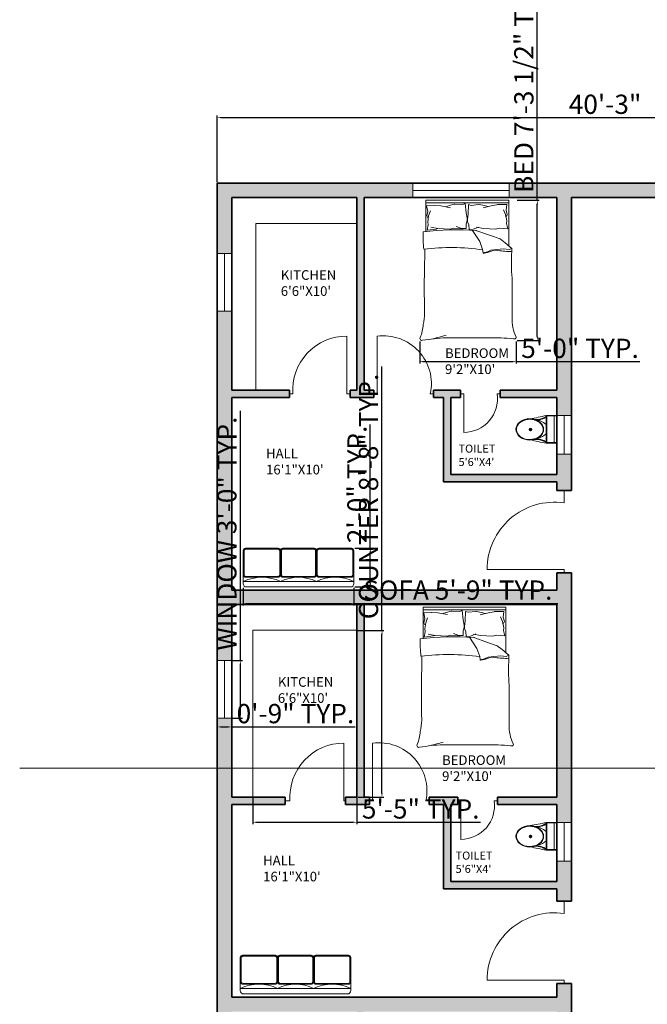
# Model space of a CAD drawing. Units: inches. Extents: x 1266 to 2869, y -408 to 3241.
# Tile 8 of 11: x 2029 to 2420, y 1767 to 2380. Entities that reach past the tile are written whole.
import ezdxf

# ---------------------------------------------------------------- set-up
doc = ezdxf.new("R2010")
doc.units = ezdxf.units.IN
for name, color, linetype, lineweight in [('A-ANNO-DIMS', 2, 'Continuous', 18), ('A-ANNO-SYMB', 7, 'Continuous', 18), ('A-AREA-IDEN', 7, 'Continuous', 18), ('A-DOOR', 4, 'Continuous', 18), ('A-FLOR-CASE', 9, 'Continuous', 18), ('A-FLOR-FIXT', 9, 'Continuous', 18), ('A-FURN', 8, 'Continuous', 18), ('A-GLAZ', 4, 'Continuous', 18), ('A-WALL', 7, 'Continuous', 35), ('A-WALL-PATT', 251, 'Continuous', 13)]:
    doc.layers.add(name, color=color, linetype=linetype, lineweight=lineweight)
doc.styles.get("Standard").update_dxf_attribs({"font": 'arial.ttf'})
doc.dimstyles.new('ISO-25', dxfattribs={"dimtxt": 12, "dimasz": 2.5, "dimexe": 1.25, "dimexo": 0.625, "dimtad": 1, "dimdec": 0, "dimlunit": 3, "dimtxsty": 'Standard', "dimcen": 2.5, "dimadec": 0, "dimazin": 0, "dimtfac": 1, "dimtdec": 0, "dimtmove": 0, "dimatfit": 3, "dimfxl": 1, "dimarcsym": 0})

# ---------------------------------------------------------------- blocks, each defined once
blk = doc.blocks.new('A$C31115884')
for p, q in [((283, 498), (223, 498)), ((258, 466), (258, 523)), ((0, 200), (0, 0)), ((520, 200), (0, 200)), ((10, 190), (10, 10)), ((510, 190), (10, 190)), ((510, 10), (510, 190)), ((520, 0), (520, 200)), ((510, 54), (0, 54)), ((10, 10), (510, 10)), ((0, 0), (520, 0))]:
    blk.add_line(p, q)
blk.add_circle((256, 496), 23.6)
for centre, radius, start, end in [((2778, -205), 2807, 165.4549, 171.7133), ((-295, 403), 365, 324.2091, 9.3499), ((-295, 403), 375, 324.2091, 9.3499), ((139, 406), 293, 315.8436, 2.6563), ((806, 403), 375, 179.2036, 215.7909), ((806, 403), 365, 170.6501, 215.7909), ((3237, 905), 2807, 188.2867, 194.5451), ((384, 406), 293, 190.2774, 224.1564)]:
    blk.add_arc(centre, radius, start, end)
blk.add_ellipse((256, 510), major_axis=(0, -261), ratio=0.772727)
blk.add_open_spline([(256, 259), (263, 259), (270, 260), (288, 262), (299, 265), (320, 273), (330, 278), (350, 291), (360, 299), (378, 316), (386, 326), (402, 347), (409, 358), (421, 383), (427, 395), (436, 422), (440, 436), (445, 465), (447, 480), (448, 509), (448, 524), (445, 553), (443, 568), (436, 596), (432, 610), (422, 636), (416, 649), (402, 672), (395, 683), (379, 703), (370, 712), (351, 728), (341, 735), (321, 746), (310, 751), (289, 757), (278, 759), (256, 761), (245, 761), (223, 757), (212, 754), (191, 746), (181, 741), (161, 728), (151, 720), (133, 703), (125, 693), (110, 672), (103, 660), (90, 636), (85, 623), (76, 596), (72, 582), (67, 553), (66, 538), (64, 509), (65, 494), (68, 465), (70, 450), (77, 422), (81, 408), (91, 382), (97, 370), (111, 346), (118, 335), (135, 316), (144, 307), (162, 291), (172, 284), (193, 273), (203, 269), (225, 262), (236, 260), (250, 259), (253, 259), (256, 259)], degree=3, knots=[0, 0, 0, 0, 0.110105, 0.110105, 0.285049, 0.285049, 0.459994, 0.459994, 0.634938, 0.634938, 0.809882, 0.809882, 0.984827, 0.984827, 1.159771, 1.159771, 1.334715, 1.334715, 1.50966, 1.50966, 1.684604, 1.684604, 1.859549, 1.859549, 2.034493, 2.034493, 2.209437, 2.209437, 2.384382, 2.384382, 2.559326, 2.559326, 2.73427, 2.73427, 2.909215, 2.909215, 3.084159, 3.084159, 3.259103, 3.259103, 3.434048, 3.434048, 3.608992, 3.608992, 3.783936, 3.783936, 3.958881, 3.958881, 4.133825, 4.133825, 4.30877, 4.30877, 4.483714, 4.483714, 4.658658, 4.658658, 4.833603, 4.833603, 5.008547, 5.008547, 5.183491, 5.183491, 5.358436, 5.358436, 5.53338, 5.53338, 5.708324, 5.708324, 5.883269, 5.883269, 6.058213, 6.058213, 6.233158, 6.233158, 6.283185, 6.283185, 6.283185, 6.283185])
blk = doc.blocks.new('*D4')
at = {"layer": 'A-ANNO-DIMS', "color": 0, "lineweight": -2, "transparency": 16777216}
for p, q in [((2152.45, 2278.97), (2152.45, 2320.42)), ((2154.95, 2319.17), (2632.95, 2319.17)), ((2635.45, 2278.97), (2635.45, 2320.42))]:
    blk.add_line(p, q, dxfattribs=at)
at = {"layer": 'A-ANNO-DIMS', "color": 0, "transparency": 16777216}
for points in [[(2154.95, 2319.59), (2154.95, 2318.76), (2152.45, 2319.17)], [(2632.95, 2319.59), (2632.95, 2318.76), (2635.45, 2319.17)]]:
    blk.add_solid(points, dxfattribs=at)
at = {"layer": 'Defpoints', "color": 0, "transparency": 16777216}
for p in [(2635.45, 2319.17), (2152.45, 2278.35), (2635.45, 2278.35)]:
    blk.add_point(p, dxfattribs=at)
at = {"layer": 'A-ANNO-DIMS', "color": 0, "transparency": 16777216, "insert": (2393.95, 2325.93), "char_height": 12, "attachment_point": 5}
blk.add_mtext('40\'-3"', dxfattribs=at)
blk = doc.blocks.new('BED-DOUBLE')
for p, q in [((3.76, 67.77), (3.76, 87.35)), ((3.76, 87.35), (55.42, 87.35)), ((55.42, 87.35), (55.42, 58.59)), ((3.76, 85.69), (55.42, 85.69)), ((4.21, 83.74), (8.84, 84.1)), ((4.21, 83.77), (4.84, 80.33)), ((4.84, 80.33), (4.37, 77.51)), ((5.46, 77.67), (6.55, 80.64)), ((8.84, 84.1), (8.96, 84.08)), ((8.96, 84.08), (13.09, 83.77)), ((13.09, 83.77), (19.03, 82.67)), ((16.06, 83.3), (18.25, 84.08)), ((18.25, 84.08), (21.37, 84.86)), ((21.37, 84.86), (21.72, 84.86)), ((21.72, 84.86), (26.53, 84.7)), ((26.53, 84.7), (28.09, 85.33)), ((28.09, 85.33), (28.71, 79.55)), ((30.24, 84.66), (29.98, 78.85)), ((31.84, 84.13), (30.24, 84.66)), ((36.63, 84.59), (31.84, 84.13)), ((36.98, 84.61), (36.63, 84.59)), ((40.14, 84.02), (36.98, 84.61)), ((45.31, 84.03), (39.45, 82.57)), ((42.38, 83.38), (40.14, 84.02)), ((49.42, 84.6), (45.31, 84.03)), ((54.17, 84.59), (48.33, 84.69)), ((48.33, 84.69), (49.42, 84.6)), ((53.3, 78.43), (52.03, 81.32)), ((54.17, 84.59), (53.76, 81.12)), ((53.76, 81.12), (54.41, 78.34)), ((4.37, 77.51), (4.99, 76.42)), ((4.84, 73.76), (5.46, 77.67)), ((5.15, 72.04), (4.84, 73.76)), ((28.71, 79.55), (29.34, 76.11)), ((29.34, 74.7), (28.71, 72.67)), ((29.34, 76.11), (29.34, 74.7)), ((29.98, 78.85), (29.57, 75.38)), ((29.57, 75.38), (29.66, 73.97)), ((29.66, 73.97), (30.41, 71.98)), ((54.17, 74.56), (53.3, 78.43)), ((54.41, 78.34), (53.85, 77.21)), ((53.97, 72.83), (54.17, 74.56)), ((4.52, 68.61), (5.15, 72.04)), ((10.03, 69.39), (4.52, 68.61)), ((6.9, 70.46), (11.26, 69.74)), ((11.26, 69.74), (10.03, 69.39)), ((11.26, 69.74), (18.84, 69.27)), ((18.84, 69.27), (20.95, 69.87)), ((20.95, 69.87), (26.5, 69.44)), ((26.06, 69.77), (22.66, 70.95)), ((28.71, 69.77), (26.06, 69.77)), ((28.71, 72.67), (28.71, 69.77)), ((30.41, 71.98), (30.59, 69.09)), ((30.59, 69.09), (33.24, 69.26)), ((32.71, 68.56), (37.24, 61.54)), ((33.24, 69.26), (36.56, 70.64)), ((43.94, 65.39), (34.92, 68.56)), ((35.2, 70.46), (39.56, 69.74)), ((39.56, 69.74), (47.14, 69.27)), ((47.14, 69.27), (49.26, 69.87)), ((49.26, 69.87), (54.81, 69.44)), ((54.81, 69.44), (53.97, 72.83)), ((37.24, 61.54), (39.08, 56.69)), ((49.96, 63.21), (43.94, 65.39)), ((53.15, 60.87), (49.96, 63.21)), ((39.08, 56.69), (39.42, 54.51)), ((42.1, 55.18), (44.27, 56.19)), ((44.27, 56.19), (47.96, 56.69)), ((47.96, 56.69), (52.14, 57.02)), ((52.14, 57.02), (55.49, 56.69)), ((57.15, 57.36), (53.15, 60.87)), ((55.49, 56.69), (57.15, 57.36)), ((57.24, 55.47), (57.15, 57.36, 4.18)), ((39.42, 54.51), (42.1, 55.18)), ((16.28, 1.69), (42.89, 1.69))]:
    blk.add_line(p, q)
for centre, radius, start, end in [((92.06, 65.63), 90.06, 178.72178, 185.60397), ((23.09, -109.45), 178.34, 86.08655, 96.78213), ((19.19, -81.63), 139.47, 81.78449, 96.90062), ((-180.86, 53.65), 183.89, 358.4762, 1.00819), ((33.68, 85.75), 32.06, 280.66171, 289.88058), ((47.29, 49.44), 6.73, 78.6608, 113.73842), ((55.49, 94.55), 39.11, 259.87628, 272.56571), ((197.03, 48.09), 139.99, 176.97912, 183.83645), ((39.6, 54.45), 0.199, 160.24637, 271.13765), ((524.11, 32.64), 521.39, 178.22771, 181.71854), ((-4874.07, 14.03), 4931.49, 0.00217, 0.28689), ((-29.08, 17.61), 32.04, 346.06484, 358.91125), ((82.33, 13.12), 24.93, 177.47136, 206.46809), ((-23.41, 11.38), 25.47, 337.97508, 356.652), ((1.18, 1.17), 1.18, 146.17358, 293.47814), ((23.16, -129.76), 131.62, 92.99578, 99.40907), ((-18.62, 112.98), 115.08, 283.38322, 287.70533), ((44.49, -142.13), 143.82, 84.4998, 90.63509), ((58.82, 2.09), 1.19, 242.65876, 356.02002)]:
    blk.add_arc(centre, radius, start, end)
blk = doc.blocks.new('SOFA-3-SEAT-2')
for points in [[(0, 22.36), (0, 7.74, 0.414214), (1.72, 6.02), (21.5, 6.02, 0.414214), (23.22, 7.74), (23.22, 22.36, 0.414214), (21.5, 24.08), (1.72, 24.08, 0.414214)], [(0.52, 22.36), (0.52, 7.74, 0.414214), (1.72, 6.53), (21.5, 6.53, 0.414214), (22.7, 7.74), (22.7, 22.36, 0.414214), (21.5, 23.56), (1.72, 23.56, 0.414214)], [(45.57, 22.36), (45.57, 7.74, -0.414214), (43.85, 6.02), (24.94, 6.02, -0.414214), (23.22, 7.74), (23.22, 22.36, -0.414214), (24.94, 24.08), (43.85, 24.08, -0.414214)], [(45.06, 22.36), (45.06, 7.74, -0.414214), (43.85, 6.53), (24.94, 6.53, -0.414214), (23.73, 7.74), (23.73, 22.36, -0.414214), (24.94, 23.56), (43.85, 23.56, -0.414214)], [(45.57, 22.36), (45.57, 7.74, 0.414214), (47.29, 6.02), (67.07, 6.02, 0.414214), (68.79, 7.74), (68.79, 22.36, 0.414214), (67.07, 24.08), (47.29, 24.08, 0.414214)], [(46.09, 22.36), (46.09, 7.74, 0.414214), (47.29, 6.53), (67.07, 6.53, 0.414214), (68.27, 7.74), (68.27, 22.36, 0.414214), (67.07, 23.56), (47.29, 23.56, 0.414214)]]:
    blk.add_lwpolyline(points, format="xyb", close=True)
at = {"ltscale": 0.03}
blk.add_lwpolyline([(21.82, 24.08), (1.38, 24.08, 0.414214), (0, 22.7), (0, 2.06, 0.414214), (2.06, 0), (66.73, 0, 0.414214), (68.79, 2.06), (68.79, 22.7, 0.414214), (67.41, 24.08), (46.97, 24.08, 0.414214), (45.59, 22.7, -1), (45.56, 22.7, 0.414214), (44.18, 24.08), (24.61, 24.08, 0.414214), (23.23, 22.7, -1), (23.2, 22.7, 0.414214)], format="xyb", close=True, dxfattribs=at)
blk.add_lwpolyline([(0, 3.44), (68.79, 3.44)])
for centre, radius, start, end in [((11.61, -21.35), 27.38, 64.91063, 115.08937), ((34.4, -19.35), 25.38, 63.869, 116.131), ((57.18, -21.07), 27.12, 64.65382, 115.34618)]:
    blk.add_arc(centre, radius, start, end)
blk = doc.blocks.new('DOOR-KITCHEN-L')
for p, q in [((35.61, 0), (35.61, 36)), ((0, 0), (2, 0)), ((37.61, 0), (35.61, 0))]:
    blk.add_line(p, q)
blk.add_arc((35.61, 2.31), 33.69, 90, 183.92625)
blk = doc.blocks.new('DOOR-BEDROOM-L')
for p, q in [((2, 0), (2, 36)), ((0, 0), (2, 0)), ((37.12, 0.11), (35.12, 0.11))]:
    blk.add_line(p, q)
blk.add_arc((5.98, 6.45), 29.82, 347.72217, 97.67592)
blk = doc.blocks.new('DOOR-BATH-L')
for p, q in [((0, 24), (2, 24)), ((2, 24), (2, 0)), ((24.7, 24), (22.7, 24))]:
    blk.add_line(p, q)
blk.add_arc((2, 20.92), 20.92, 270, 8.45113)
blk = doc.blocks.new('DOOR-ENTRY-L')
for p, q in [((48, 51.27), (48, 45.59)), ((48, 45.59), (48, 43.59)), ((12, 2), (0, 2)), ((48, 2), (12, 2)), ((48, 0), (48, 2))]:
    blk.add_line(p, q)
blk.add_arc((42.02, 2), 42.02, 81.81164, 180)
blk = doc.blocks.new('WIN-PLAN-60')
for p, q in [((0, 9), (0, 0)), ((60, 4.5), (60, 9)), ((60, 9), (60, 0)), ((0, 4.5), (60, 4.5)), ((0, 0), (0, 4.5))]:
    blk.add_line(p, q)
blk = doc.blocks.new('WIN-PLAN-36')
for p, q in [((0, 36), (9, 36)), ((4.5, 36), (4.5, 0)), ((9, 36), (4.5, 36)), ((4.5, 0), (0, 0)), ((0, 0), (9, 0))]:
    blk.add_line(p, q)
blk = doc.blocks.new('WIN-PLAN-36-2')
for p, q in [((0, 36), (9, 36)), ((4.5, 36), (4.5, 0)), ((9, 36), (4.5, 36)), ((2.69, 0), (0, 0)), ((0, 0), (9, 0))]:
    blk.add_line(p, q)
blk = doc.blocks.new('WIN-PLAN-24-2')
for p, q in [((0, 24), (9, 24)), ((4.5, 24), (4.5, 0)), ((9, 24), (4.5, 24)), ((4.5, 0), (0, 0)), ((0, 0), (9, 0))]:
    blk.add_line(p, q)
blk = doc.blocks.new('WIN-PLAN-24-3')
for p, q in [((0, 24), (9, 24)), ((4.5, 24), (4.5, 0)), ((9, 24), (4.5, 24)), ((2.69, 0), (0, 0)), ((0, 0), (9, 0))]:
    blk.add_line(p, q)
blk = doc.blocks.new('COUNTER-KITCHEN-2')
for p, q in [((0, 0), (0, 103.95)), ((0, 103.95), (63, 103.95))]:
    blk.add_line(p, q)
blk = doc.blocks.new('COUNTER-KITCHEN-3')
for p, q in [((0, 0), (0, 103.95)), ((0, 103.95), (64.81, 103.95))]:
    blk.add_line(p, q)
blk = doc.blocks.new('*D39')
at = {"layer": 'A-ANNO-DIMS', "color": 0, "lineweight": -2, "transparency": 16777216}
for p, q in [((2351.77, 2267.74), (2351.77, 2411.2)), ((2339.28, 2267.74), (2353.02, 2267.74)), ((2351.77, 2182.78), (2351.77, 2265.24)), ((2339.28, 2180.28), (2353.02, 2180.28))]:
    blk.add_line(p, q, dxfattribs=at)
at = {"layer": 'A-ANNO-DIMS', "color": 0, "transparency": 16777216}
for points in [[(2351.36, 2265.24), (2352.19, 2265.24), (2351.77, 2267.74)], [(2351.36, 2182.78), (2352.19, 2182.78), (2351.77, 2180.28)]]:
    blk.add_solid(points, dxfattribs=at)
at = {"layer": 'Defpoints', "color": 0, "transparency": 16777216}
for p in [(2338.65, 2267.74), (2351.77, 2267.74), (2338.65, 2180.28)]:
    blk.add_point(p, dxfattribs=at)
at = {"layer": 'A-ANNO-DIMS', "color": 0, "transparency": 16777216, "insert": (2344.94, 2340.72), "char_height": 12, "attachment_point": 5, "rotation": 90}
blk.add_mtext('BED 7\'-3 1/2" TYP.', dxfattribs=at)
blk = doc.blocks.new('*D40')
at = {"layer": 'A-ANNO-DIMS', "color": 0, "lineweight": -2, "transparency": 16777216}
for p, q in [((2278.55, 2179.65), (2278.55, 2165.91)), ((2338.65, 2179.65), (2338.65, 2165.91)), ((2281.05, 2167.16), (2336.15, 2167.16)), ((2338.65, 2167.16), (2415.55, 2167.16))]:
    blk.add_line(p, q, dxfattribs=at)
at = {"layer": 'A-ANNO-DIMS', "color": 0, "transparency": 16777216}
for points in [[(2281.05, 2167.58), (2281.05, 2166.74), (2278.55, 2167.16)], [(2336.15, 2167.58), (2336.15, 2166.74), (2338.65, 2167.16)]]:
    blk.add_solid(points, dxfattribs=at)
at = {"layer": 'Defpoints', "color": 0, "transparency": 16777216}
for p in [(2278.55, 2180.28), (2338.65, 2180.28), (2338.65, 2167.16)]:
    blk.add_point(p, dxfattribs=at)
at = {"layer": 'A-ANNO-DIMS', "color": 0, "transparency": 16777216, "insert": (2378.35, 2173.91), "char_height": 12, "attachment_point": 5}
blk.add_mtext('5\'-0" TYP.', dxfattribs=at)
blk = doc.blocks.new('*D69')
at = {"layer": 'A-ANNO-DIMS', "color": 0, "lineweight": -2, "transparency": 16777216}
for p, q in [((2168.66, 2026.17), (2168.66, 2015.23)), ((2237.45, 2026.17), (2237.45, 2015.23)), ((2171.16, 2016.48), (2234.95, 2016.48)), ((2237.45, 2016.48), (2364.59, 2016.48))]:
    blk.add_line(p, q, dxfattribs=at)
at = {"layer": 'A-ANNO-DIMS', "color": 0, "transparency": 16777216}
for points in [[(2171.16, 2016.9), (2171.16, 2016.06), (2168.66, 2016.48)], [(2234.95, 2016.9), (2234.95, 2016.06), (2237.45, 2016.48)]]:
    blk.add_solid(points, dxfattribs=at)
at = {"layer": 'Defpoints', "color": 0, "transparency": 16777216}
for p in [(2168.66, 2026.8), (2237.45, 2026.8), (2237.45, 2016.48)]:
    blk.add_point(p, dxfattribs=at)
at = {"layer": 'A-ANNO-DIMS', "color": 0, "transparency": 16777216, "insert": (2302.27, 2023.31), "char_height": 12, "attachment_point": 5}
blk.add_mtext('SOFA 5\'-9" TYP.', dxfattribs=at)
blk = doc.blocks.new('*D70')
at = {"layer": 'A-ANNO-DIMS', "color": 0, "lineweight": -2, "transparency": 16777216}
for p, q in [((2247.77, 2050.88), (2247.77, 2127.98)), ((2238.07, 2050.88), (2249.02, 2050.88)), ((2247.77, 2029.3), (2247.77, 2048.38)), ((2238.07, 2026.8), (2249.02, 2026.8))]:
    blk.add_line(p, q, dxfattribs=at)
at = {"layer": 'A-ANNO-DIMS', "color": 0, "transparency": 16777216}
for points in [[(2247.35, 2048.38), (2248.18, 2048.38), (2247.77, 2050.88)], [(2247.35, 2029.3), (2248.18, 2029.3), (2247.77, 2026.8)]]:
    blk.add_solid(points, dxfattribs=at)
at = {"layer": 'Defpoints', "color": 0, "transparency": 16777216}
for p in [(2237.45, 2050.88), (2247.77, 2050.88), (2237.45, 2026.8)]:
    blk.add_point(p, dxfattribs=at)
at = {"layer": 'A-ANNO-DIMS', "color": 0, "transparency": 16777216, "insert": (2241.02, 2090.68), "char_height": 12, "attachment_point": 5, "rotation": 90}
blk.add_mtext('2\'-0" TYP.', dxfattribs=at)
blk = doc.blocks.new('*D75')
at = {"layer": 'A-ANNO-DIMS', "color": 0, "lineweight": -2, "transparency": 16777216}
for p, q in [((2166.85, 1981.02), (2166.85, 2136.62)), ((2162.08, 1981.02), (2168.1, 1981.02)), ((2166.85, 1947.52), (2166.85, 1978.52)), ((2162.08, 1945.02), (2168.1, 1945.02))]:
    blk.add_line(p, q, dxfattribs=at)
at = {"layer": 'A-ANNO-DIMS', "color": 0, "transparency": 16777216}
for points in [[(2166.43, 1978.52), (2167.27, 1978.52), (2166.85, 1981.02)], [(2166.43, 1947.52), (2167.27, 1947.52), (2166.85, 1945.02)]]:
    blk.add_solid(points, dxfattribs=at)
at = {"layer": 'Defpoints', "color": 0, "transparency": 16777216}
for p in [(2161.45, 1981.02), (2166.85, 1981.02), (2161.45, 1945.02)]:
    blk.add_point(p, dxfattribs=at)
at = {"layer": 'A-ANNO-DIMS', "color": 0, "transparency": 16777216, "insert": (2160.01, 2060.07), "char_height": 12, "attachment_point": 5, "rotation": 90}
blk.add_mtext('WINDOW 3\'-0" TYP.', dxfattribs=at)
blk = doc.blocks.new('*D76')
at = {"layer": 'A-ANNO-DIMS', "color": 0, "lineweight": -2, "transparency": 16777216}
for p, q in [((2152.45, 1944.4), (2152.45, 1938.37)), ((2161.45, 1944.4), (2161.45, 1938.37)), ((2154.95, 1939.62), (2158.95, 1939.62)), ((2161.45, 1939.62), (2238.35, 1939.62))]:
    blk.add_line(p, q, dxfattribs=at)
at = {"layer": 'A-ANNO-DIMS', "color": 0, "transparency": 16777216}
for points in [[(2154.95, 1940.04), (2154.95, 1939.21), (2152.45, 1939.62)], [(2158.95, 1940.04), (2158.95, 1939.21), (2161.45, 1939.62)]]:
    blk.add_solid(points, dxfattribs=at)
at = {"layer": 'Defpoints', "color": 0, "transparency": 16777216}
for p in [(2152.45, 1945.02), (2161.45, 1945.02), (2161.45, 1939.62)]:
    blk.add_point(p, dxfattribs=at)
at = {"layer": 'A-ANNO-DIMS', "color": 0, "transparency": 16777216, "insert": (2201.15, 1946.38), "char_height": 12, "attachment_point": 5}
blk.add_mtext('0\'-9" TYP.', dxfattribs=at)
blk = doc.blocks.new('*D79')
at = {"layer": 'A-ANNO-DIMS', "color": 0, "lineweight": -2, "transparency": 16777216}
for p, q in [((2255.04, 1999.79), (2255.04, 2164.1)), ((2240.08, 1999.79), (2256.29, 1999.79)), ((2255.04, 1898.35), (2255.04, 1997.29)), ((2240.08, 1895.85), (2256.29, 1895.85))]:
    blk.add_line(p, q, dxfattribs=at)
at = {"layer": 'A-ANNO-DIMS', "color": 0, "transparency": 16777216}
for points in [[(2254.63, 1997.29), (2255.46, 1997.29), (2255.04, 1999.79)], [(2254.63, 1898.35), (2255.46, 1898.35), (2255.04, 1895.85)]]:
    blk.add_solid(points, dxfattribs=at)
at = {"layer": 'Defpoints', "color": 0, "transparency": 16777216}
for p in [(2239.45, 1999.79), (2255.04, 1999.79), (2239.45, 1895.85)]:
    blk.add_point(p, dxfattribs=at)
at = {"layer": 'A-ANNO-DIMS', "color": 0, "transparency": 16777216, "insert": (2248.21, 2083.2), "char_height": 12, "attachment_point": 5, "rotation": 90}
blk.add_mtext('COUNTER 8\'-8" TYP.', dxfattribs=at)
blk = doc.blocks.new('*D80')
at = {"layer": 'A-ANNO-DIMS', "color": 0, "lineweight": -2, "transparency": 16777216}
for p, q in [((2174.64, 1895.22), (2174.64, 1879)), ((2239.45, 1895.22), (2239.45, 1879)), ((2177.14, 1880.25), (2236.95, 1880.25)), ((2239.45, 1880.25), (2316.35, 1880.25))]:
    blk.add_line(p, q, dxfattribs=at)
at = {"layer": 'A-ANNO-DIMS', "color": 0, "transparency": 16777216}
for points in [[(2177.14, 1880.67), (2177.14, 1879.84), (2174.64, 1880.25)], [(2236.95, 1880.67), (2236.95, 1879.84), (2239.45, 1880.25)]]:
    blk.add_solid(points, dxfattribs=at)
at = {"layer": 'Defpoints', "color": 0, "transparency": 16777216}
for p in [(2174.64, 1895.85), (2239.45, 1895.85), (2239.45, 1880.25)]:
    blk.add_point(p, dxfattribs=at)
at = {"layer": 'A-ANNO-DIMS', "color": 0, "transparency": 16777216, "insert": (2279.15, 1886.98), "char_height": 12, "attachment_point": 5}
blk.add_mtext('5\'-5" TYP.', dxfattribs=at)

msp = doc.modelspace()

# ---------------------------------------------------------------- hatches: boundary and pattern name
at = {"layer": 'A-WALL-PATT'}
h = msp.add_hatch(color=256, dxfattribs=at)
h.dxf.hatch_style = 1
h.paths.add_polyline_path([(2161.45, 2269.35), (2239.45, 2269.35), (2239.45, 2149.35), (2235.18, 2149.35), (2235.18, 2144.85), (2243.95, 2144.85), (2249.99, 2144.85), (2249.99, 2146.74), (2249.99, 2149.35), (2243.95, 2149.35), (2243.95, 2269.35), (2274.21, 2269.35), (2274.21, 2273.85), (2274.21, 2278.35), (2152.45, 2278.35), (2152.45, 2234.52), (2161.45, 2234.52)])
h.paths.add_polyline_path([(2550.01, 2278.35), (2424.95, 2278.35), (2372.95, 2278.35), (2334.21, 2278.35), (2334.21, 2269.35), (2363.95, 2269.35), (2363.95, 2149.35), (2328.7, 2149.35), (2328.7, 2144.85), (2363.95, 2144.85), (2363.95, 2133.61), (2372.95, 2133.61), (2372.95, 2269.35), (2424.95, 2269.35), (2424.95, 2234.52), (2433.95, 2234.52), (2433.95, 2269.35), (2511.95, 2269.35), (2511.95, 2149.35), (2504.09, 2149.35), (2504.09, 2144.85), (2520.49, 2144.85), (2520.49, 2149.35), (2516.45, 2149.35), (2516.45, 2269.35), (2550.01, 2269.35), (2550.01, 2273.85)])
h.paths.add_polyline_path([(2635.45, 2278.35), (2610.01, 2278.35), (2610.01, 2269.35), (2626.45, 2269.35), (2626.45, 2149.35), (2588.98, 2149.35), (2588.98, 2144.85), (2626.45, 2144.85), (2626.45, 2133.61), (2635.45, 2133.61)])
h.paths.add_polyline_path([(2560.45, 2144.85), (2565.84, 2144.85), (2565.84, 2149.35), (2552.33, 2149.35), (2552.33, 2144.85), (2555.95, 2144.85), (2555.95, 2092.35), (2626.45, 2092.35), (2626.45, 2086.89), (2626.45, 2024.85), (2610.01, 2024.85), (2610.01, 2015.85), (2626.45, 2015.85), (2626.45, 1895.85), (2589.21, 1895.85), (2589.21, 1891.35), (2626.45, 1891.35), (2626.45, 1880.11), (2635.45, 1880.11), (2635.45, 2086.89), (2635.45, 2109.61), (2626.45, 2109.61), (2626.45, 2096.85), (2560.45, 2096.85)])
h.paths.add_polyline_path([(2433.95, 2198.52), (2424.95, 2198.52), (2424.95, 2086.89), (2433.95, 2086.89), (2433.95, 2144.85), (2470.3, 2144.85), (2470.3, 2149.35), (2433.95, 2149.35)])
h.paths.add_polyline_path([(2372.95, 2109.61), (2363.95, 2109.61), (2363.95, 2096.85), (2297.95, 2096.85), (2297.95, 2144.85), (2304, 2144.85), (2304, 2149.35), (2293.45, 2149.35), (2287.11, 2149.35), (2287.11, 2144.85), (2293.45, 2144.85), (2293.45, 2092.35), (2363.95, 2092.35), (2363.95, 2086.89), (2372.95, 2086.89)], flags=17)
h.paths.add_polyline_path([(2161.45, 2144.85), (2197.56, 2144.85), (2197.56, 2149.35), (2161.45, 2149.35), (2161.45, 2198.52), (2152.45, 2198.52), (2152.45, 1981.02), (2161.45, 1981.02), (2161.45, 2015.85), (2363.95, 2015.85), (2363.95, 1895.85), (2326.89, 1895.85), (2326.89, 1891.35), (2363.95, 1891.35), (2363.95, 1880.11), (2372.95, 1880.11), (2372.95, 2035.62), (2363.95, 2035.62), (2363.95, 2024.85), (2161.45, 2024.85)])
h.paths.add_polyline_path([(2161.45, 1691.52), (2152.45, 1691.52), (2152.45, 1474.02), (2161.45, 1474.02)])
h.paths.add_polyline_path([(2194.79, 1895.85), (2161.45, 1895.85), (2161.45, 1945.02), (2152.45, 1945.02), (2152.45, 1727.52), (2161.45, 1727.52), (2161.45, 1762.35), (2363.95, 1762.35), (2363.95, 1642.35), (2328.7, 1642.35), (2328.7, 1637.85), (2363.95, 1637.85), (2363.95, 1589.85), (2297.95, 1589.85), (2297.95, 1637.85), (2303.95, 1637.85), (2303.95, 1642.35), (2287.64, 1642.35), (2287.64, 1637.85), (2293.45, 1637.85), (2293.45, 1585.35), (2363.95, 1585.35), (2363.95, 1579.45), (2372.95, 1579.45), (2372.95, 1779.84), (2363.95, 1779.84), (2363.95, 1771.35), (2161.45, 1771.35), (2161.45, 1891.35), (2194.79, 1891.35)])
h.paths.add_polyline_path([(2243.95, 2015.85), (2239.45, 2015.85), (2239.45, 1895.85), (2232.4, 1895.85), (2232.4, 1891.35), (2247.22, 1891.35), (2247.22, 1895.85), (2243.95, 1895.85)], flags=17)
h.paths.add_polyline_path([(2302.19, 1895.85), (2284.34, 1895.85), (2284.34, 1891.35), (2293.45, 1891.35), (2293.45, 1838.85), (2363.95, 1838.85), (2363.95, 1831.11), (2372.95, 1831.11), (2372.95, 1856.11), (2363.95, 1856.11), (2363.95, 1843.35), (2297.95, 1843.35), (2297.95, 1891.35), (2302.19, 1891.35)], flags=17)
h.paths.add_polyline_path([(2243.95, 1762.35), (2239.45, 1762.35), (2239.45, 1642.35), (2235.18, 1642.35), (2235.18, 1637.85), (2249.99, 1637.85), (2249.99, 1642.35), (2243.95, 1642.35)], flags=17)
h.paths.add_polyline_path([(2197.56, 1642.35), (2161.45, 1642.35), (2161.45, 1637.85), (2197.56, 1637.85)], flags=17)
h.paths.add_polyline_path([(2363.95, 1517.85), (2161.45, 1517.85), (2161.45, 1508.85), (2239.45, 1508.85), (2239.45, 1388.85), (2243.95, 1388.85), (2243.95, 1508.85), (2363.95, 1508.85)])
h.paths.add_polyline_path([(2372.95, 1528.18), (2363.95, 1528.18), (2363.95, 1323.21), (2372.95, 1323.21)])
h.paths.add_polyline_path([(2372.95, 1271.94), (2363.95, 1271.94), (2363.95, 1264.35), (2161.45, 1264.35), (2161.45, 1283.77), (2156.95, 1283.77), (2152.45, 1283.77), (2152.45, 1255.35), (2156.95, 1255.35), (2372.95, 1255.35)])
h.paths.add_polyline_path([(2161.45, 1438.02), (2152.45, 1438.02), (2152.45, 1319.77), (2161.45, 1319.77)])
h.paths.add_polyline_path([(2550.01, 1513.35), (2550.01, 1517.85), (2433.95, 1517.85), (2433.95, 1528.62), (2424.95, 1528.62), (2424.95, 1474.02), (2433.95, 1474.02), (2433.95, 1508.85), (2511.95, 1508.85), (2511.95, 1388.85), (2504.09, 1388.85), (2504.09, 1384.35), (2520.49, 1384.35), (2520.49, 1388.85), (2516.45, 1388.85), (2516.45, 1508.85), (2550.01, 1508.85)])
h.paths.add_polyline_path([(2635.45, 1602.61), (2626.45, 1602.61), (2626.45, 1517.85), (2610.01, 1517.85), (2610.01, 1508.85), (2626.45, 1508.85), (2626.45, 1388.85), (2588.98, 1388.85), (2588.98, 1384.35), (2626.45, 1384.35), (2626.45, 1373.11), (2635.45, 1373.11)])
h.paths.add_polyline_path([(2635.45, 1349.11), (2626.45, 1349.11), (2626.45, 1336.35), (2560.45, 1336.35), (2560.45, 1384.35), (2565.84, 1384.35), (2565.84, 1388.85), (2552.33, 1388.85), (2552.33, 1384.35), (2555.95, 1384.35), (2555.95, 1331.85), (2626.45, 1331.85), (2626.45, 1315.59), (2635.45, 1315.59)])
h.paths.add_polyline_path([(2635.45, 1279.59), (2630.95, 1279.59), (2626.45, 1279.59), (2626.45, 1264.35), (2433.95, 1264.35), (2433.95, 1275.12), (2424.95, 1275.12), (2424.95, 1255.35), (2635.45, 1255.35)])
h.paths.add_polyline_path([(2433.95, 1438.02), (2424.95, 1438.02), (2424.95, 1326.39), (2433.95, 1326.39)])
h.paths.add_polyline_path([(2470.3, 1388.85), (2433.95, 1388.85), (2433.95, 1384.35), (2470.3, 1384.35)], flags=0)

# ---------------------------------------------------------------- linework, layer by layer
at = {"layer": 'A-ANNO-SYMB'}
msp.add_line((2029.46, 1914.02), (2745.24, 1914.02), dxfattribs=at)
at = {"layer": 'A-DOOR'}
for p, q in [((2231.36, 1893.6), (2231.36, 1929.6)), ((2194.79, 1893.6), (2196.79, 1893.6)), ((2195.75, 1893.6), (2197.75, 1893.6)), ((2232.4, 1893.6), (2231.36, 1893.6)), ((2232.4, 1893.6), (2231.36, 1893.6))]:
    msp.add_line(p, q, dxfattribs=at)
msp.add_arc((2231.36, 1895.9), 33.69, 90, 183.92625, dxfattribs=at)
at = {"layer": 'A-FURN'}
for points in [[(2166.84, 1795.66), (2166.84, 1781.04, 0.414214), (2168.56, 1779.32), (2188.34, 1779.32, 0.414214), (2190.06, 1781.04), (2190.06, 1795.66, 0.414214), (2188.34, 1797.38), (2168.56, 1797.38, 0.414214)], [(2212.42, 1795.66), (2212.42, 1781.04, -0.414214), (2210.7, 1779.32), (2191.78, 1779.32, -0.414214), (2190.06, 1781.04), (2190.06, 1795.66, -0.414214), (2191.78, 1797.38), (2210.7, 1797.38, -0.414214)], [(2212.42, 1795.66), (2212.42, 1781.04, 0.414214), (2214.14, 1779.32), (2233.92, 1779.32, 0.414214), (2235.63, 1781.04), (2235.63, 1795.66, 0.414214), (2233.92, 1797.38), (2214.14, 1797.38, 0.414214)], [(2167.36, 1795.66), (2167.36, 1781.04, 0.414214), (2168.56, 1779.83), (2188.34, 1779.83, 0.414214), (2189.55, 1781.04), (2189.55, 1795.66, 0.414214), (2188.34, 1796.86), (2168.56, 1796.86, 0.414214)], [(2211.9, 1795.66), (2211.9, 1781.04, -0.414214), (2210.7, 1779.83), (2191.78, 1779.83, -0.414214), (2190.58, 1781.04), (2190.58, 1795.66, -0.414214), (2191.78, 1796.86), (2210.7, 1796.86, -0.414214)], [(2212.93, 1795.66), (2212.93, 1781.04, 0.414214), (2214.14, 1779.83), (2233.92, 1779.83, 0.414214), (2235.12, 1781.04), (2235.12, 1795.66, 0.414214), (2233.92, 1796.86), (2214.14, 1796.86, 0.414214)]]:
    msp.add_lwpolyline(points, format="xyb", close=True, dxfattribs=at)
at = {"layer": 'A-FURN', "ltscale": 0.03}
msp.add_lwpolyline([(2188.67, 1797.38), (2168.22, 1797.38, 0.414214), (2166.84, 1796), (2166.84, 1775.36, 0.414214), (2168.91, 1773.3), (2233.57, 1773.3, 0.414214), (2235.63, 1775.36), (2235.63, 1796, 0.414214), (2234.26, 1797.38), (2213.81, 1797.38, 0.414214), (2212.43, 1796, -1), (2212.4, 1796, 0.414214), (2211.03, 1797.38), (2191.45, 1797.38, 0.414214), (2190.08, 1796, -1), (2190.04, 1796, 0.414214)], format="xyb", close=True, dxfattribs=at)
at = {"layer": 'A-FURN'}
msp.add_lwpolyline([(2166.84, 1776.74), (2235.63, 1776.74)], dxfattribs=at)
for centre, radius, start, end in [((2178.45, 1751.95), 27.38, 64.91063, 115.08937), ((2201.24, 1753.95), 25.38, 63.869, 116.131), ((2224.03, 1752.23), 27.12, 64.65382, 115.34618)]:
    msp.add_arc(centre, radius, start, end, dxfattribs=at)
at = {"layer": 'A-WALL'}
for p, q in [((2152.45, 2278.35), (2152.45, 1255.35)), ((2152.45, 2278.35), (2372.95, 2278.35)), ((2372.95, 2278.35), (2424.95, 2278.35)), ((2161.45, 2269.35), (2161.45, 2149.35)), ((2161.45, 2269.35), (2239.45, 2269.35)), ((2239.45, 2269.35), (2239.45, 2149.35)), ((2243.95, 2269.35), (2243.95, 2149.35)), ((2243.95, 2269.35), (2363.95, 2269.35)), ((2363.95, 2269.35), (2363.95, 2149.35)), ((2372.95, 2269.35), (2372.95, 2086.89)), ((2424.95, 2269.35), (2372.95, 2269.35)), ((2161.45, 2149.35), (2197.56, 2149.35)), ((2197.56, 2149.35), (2197.56, 2144.85)), ((2235.18, 2149.35), (2239.45, 2149.35)), ((2235.18, 2149.35), (2235.18, 2144.85)), ((2243.95, 2149.35), (2249.99, 2149.35)), ((2249.99, 2149.35), (2249.99, 2146.74)), ((2249.99, 2146.74), (2249.99, 2144.85)), ((2293.45, 2149.35), (2287.11, 2149.35)), ((2287.11, 2149.35), (2287.11, 2144.85)), ((2293.45, 2149.35), (2304, 2149.35)), ((2304, 2149.35), (2304, 2144.85)), ((2328.7, 2149.35), (2363.95, 2149.35)), ((2328.7, 2149.35), (2328.7, 2144.85)), ((2161.45, 2144.85), (2161.45, 2024.85)), ((2161.45, 2144.85), (2197.56, 2144.85)), ((2235.18, 2144.85), (2243.95, 2144.85)), ((2249.99, 2144.85), (2243.95, 2144.85)), ((2287.11, 2144.85), (2293.45, 2144.85)), ((2293.45, 2144.85), (2293.45, 2092.35)), ((2297.95, 2144.85), (2297.95, 2096.85)), ((2297.95, 2144.85), (2304, 2144.85)), ((2328.7, 2144.85), (2363.95, 2144.85)), ((2363.95, 2144.85), (2363.95, 2096.85)), ((2293.45, 2092.35), (2363.95, 2092.35)), ((2297.95, 2096.85), (2363.95, 2096.85)), ((2363.95, 2092.35), (2363.95, 2086.89)), ((2363.95, 2086.89), (2372.95, 2086.89)), ((2363.95, 2035.62), (2363.95, 2024.85)), ((2363.95, 2035.62), (2372.95, 2035.62)), ((2372.95, 2035.62), (2372.95, 1831.11)), ((2161.45, 2024.85), (2363.95, 2024.85)), ((2161.45, 2015.85), (2161.45, 1895.85)), ((2161.45, 2015.85), (2363.95, 2015.85)), ((2239.45, 2015.85), (2239.45, 1895.85)), ((2243.95, 2015.85), (2243.95, 1895.85)), ((2363.95, 2015.85), (2363.95, 1895.85)), ((2161.45, 1895.85), (2194.79, 1895.85)), ((2194.79, 1893.6), (2194.79, 1895.85)), ((2194.79, 1895.85), (2194.79, 1891.35)), ((2232.4, 1895.85), (2239.45, 1895.85)), ((2232.4, 1895.85), (2232.4, 1891.35)), ((2243.95, 1895.85), (2247.22, 1895.85)), ((2247.22, 1893.49), (2247.22, 1895.85)), ((2247.22, 1895.85), (2247.22, 1891.35)), ((2284.34, 1893.6), (2284.34, 1895.85)), ((2284.34, 1895.85), (2284.34, 1891.35)), ((2302.19, 1895.85), (2284.34, 1895.85)), ((2302.19, 1891.35), (2302.19, 1895.85)), ((2302.19, 1895.85), (2302.19, 1895.85)), ((2326.89, 1895.85), (2363.95, 1895.85)), ((2326.89, 1893.6), (2326.89, 1895.85)), ((2326.89, 1895.85), (2326.89, 1891.35)), ((2161.45, 1891.35), (2161.45, 1771.35)), ((2161.45, 1891.35), (2194.79, 1891.35)), ((2232.4, 1891.35), (2247.22, 1891.35)), ((2284.34, 1891.35), (2293.45, 1891.35)), ((2293.45, 1891.35), (2293.45, 1838.85)), ((2297.95, 1891.35), (2297.95, 1843.35)), ((2297.95, 1891.35), (2302.19, 1891.35)), ((2326.89, 1891.35), (2363.95, 1891.35)), ((2363.95, 1891.35), (2363.95, 1843.35)), ((2297.95, 1843.35), (2363.95, 1843.35)), ((2293.45, 1838.85), (2363.95, 1838.85)), ((2363.95, 1838.85), (2363.95, 1831.11)), ((2368.45, 1831.11), (2363.95, 1831.11)), ((2363.95, 1831.11), (2372.95, 1831.11)), ((2363.95, 1779.84), (2363.95, 1771.35)), ((2363.95, 1779.84), (2363.95, 1779.84)), ((2363.95, 1779.84), (2372.95, 1779.84)), ((2372.95, 1779.84), (2372.95, 1579.45)), ((2161.45, 1771.35), (2363.95, 1771.35))]:
    msp.add_line(p, q, dxfattribs=at)

# ---------------------------------------------------------------- block references
at = {"layer": 'A-DOOR'}
for name, p in [('DOOR-BEDROOM-L', (2249.99, 2146.99)), ('DOOR-KITCHEN-L', (2197.56, 2147.1)), ('DOOR-BATH-L', (2304, 2123.1)), ('DOOR-ENTRY-L', (2320.45, 2035.62)), ('DOOR-BEDROOM-L', (2247.22, 1893.49)), ('DOOR-BATH-L', (2302.19, 1869.6)), ('DOOR-BATH-L', (2302.19, 1869.6)), ('DOOR-ENTRY-L', (2320.45, 1779.84))]:
    msp.add_blockref(name, p, dxfattribs=at)
at = {"layer": 'A-FLOR-CASE'}
for name, p in [('COUNTER-KITCHEN-2', (2176.45, 2149.35)), ('COUNTER-KITCHEN-3', (2174.64, 1895.85))]:
    msp.add_blockref(name, p, dxfattribs=at)
at = {"layer": 'A-FLOR-FIXT', "xscale": 0.0330640103915726, "yscale": 0.0330640103915726, "zscale": 0.0330640103915726, "rotation": 89.99999999999996}
for p in [(2363.95, 2116.46), (2363.95, 1862.96)]:
    msp.add_blockref('A$C31115884', p, dxfattribs=at)
at = {"layer": 'A-FURN'}
for name, p in [('BED-DOUBLE', (2278.65, 2180.39)), ('SOFA-3-SEAT-2', (2168.66, 2026.8)), ('BED-DOUBLE', (2276.83, 1926.89))]:
    msp.add_blockref(name, p, dxfattribs=at)
at = {"layer": 'A-GLAZ'}
for name, p in [('WIN-PLAN-60', (2274.21, 2269.35)), ('WIN-PLAN-36', (2152.45, 2198.52)), ('WIN-PLAN-24-2', (2363.95, 2109.61)), ('WIN-PLAN-36-2', (2152.45, 1945.02)), ('WIN-PLAN-24-3', (2363.95, 1856.11))]:
    msp.add_blockref(name, p, dxfattribs=at)

# ---------------------------------------------------------------- texts
at = {"layer": 'A-AREA-IDEN', "attachment_point": 1}
for s, width, insert, char_height in [('KITCHEN\\P6\'6"X10\'', 112.1355, (2192.04, 2224.14), 6), ('BEDROOM\\P9\'2"X10\'', 62.026, (2294.3, 2175.46), 6), ('HALL\\P16\'1"X10\'', 100.9767, (2182.86, 2112.93), 6), ('TOILET\\P5\'6"X4\'', 46.3569, (2302.69, 2115.49), 5), ('KITCHEN\\P6\'6"X10\'', 112.1355, (2190.22, 1970.64), 6), ('BEDROOM\\P9\'2"X10\'', 62.026, (2292.48, 1921.96), 6), ('HALL\\P16\'1"X10\'', 100.9767, (2181.04, 1859.43), 6), ('TOILET\\P5\'6"X4\'', 46.3569, (2300.87, 1861.99), 5)]:
    msp.add_mtext_dynamic_manual_height_columns(s, width=width, gutter_width=12.5, heights=[0], dxfattribs=dict(at, insert=insert, char_height=char_height))

# ---------------------------------------------------------------- dimensions: what is measured, and where the dimension line sits
at = {"layer": 'A-ANNO-DIMS'}
for base, p1, p2, text, picture, middle in [((2351.77, 2267.74), (2338.65, 2180.28), (2338.65, 2267.74), 'BED <> TYP.', '*D39', (2344.94, 2340.72)), ((2255.04, 1999.79), (2239.45, 1895.85), (2239.45, 1999.79), 'COUNTER <> TYP.', '*D79', (2248.21, 2083.2)), ((2166.85, 1981.02), (2161.45, 1945.02), (2161.45, 1981.02), 'WINDOW <> TYP.', '*D75', (2160.01, 2060.07)), ((2247.77, 2050.88), (2237.45, 2026.8), (2237.45, 2050.88), '<> TYP.', '*D70', (2241.02, 2090.68))]:
    dim = msp.add_linear_dim(base=base, p1=p1, p2=p2, angle=90, text=text, dimstyle='ISO-25', override={"dimdec": 1, "dimlfac": 1, "dimrnd": 0, "dimzin": 1, "dimdsep": 46, "dimlunit": 4, "dimfrac": 2}, dxfattribs=at)
    dim.commit()
    dim.dimension.update_dxf_attribs({"geometry": picture, "text_midpoint": middle})
dim = msp.add_linear_dim(base=(2635.45, 2319.17), p1=(2152.45, 2278.35), p2=(2635.45, 2278.35), dimstyle='ISO-25', override={"dimclrd": 0, "dimclre": 0, "dimclrt": 0}, dxfattribs=at)
dim.commit()
dim.dimension.update_dxf_attribs({"geometry": '*D4', "text_midpoint": (2393.95, 2319.17), "dimtype": 160})
for base, p1, p2, text, picture, middle in [((2338.65, 2167.16), (2278.55, 2180.28), (2338.65, 2180.28), '<> TYP.', '*D40', (2378.35, 2173.91)), ((2237.45, 2016.48), (2168.66, 2026.8), (2237.45, 2026.8), 'SOFA <> TYP.', '*D69', (2302.27, 2023.31)), ((2161.45, 1939.62), (2152.45, 1945.02), (2161.45, 1945.02), '<> TYP.', '*D76', (2201.15, 1946.38)), ((2239.45, 1880.25), (2174.64, 1895.85), (2239.45, 1895.85), '<> TYP.', '*D80', (2279.15, 1886.98))]:
    dim = msp.add_linear_dim(base=base, p1=p1, p2=p2, text=text, dimstyle='ISO-25', override={"dimdec": 1, "dimlfac": 1, "dimrnd": 0, "dimzin": 1, "dimdsep": 46, "dimlunit": 4, "dimfrac": 2}, dxfattribs=at)
    dim.commit()
    dim.dimension.update_dxf_attribs({"geometry": picture, "text_midpoint": middle})

doc.saveas('drawing.dxf')
